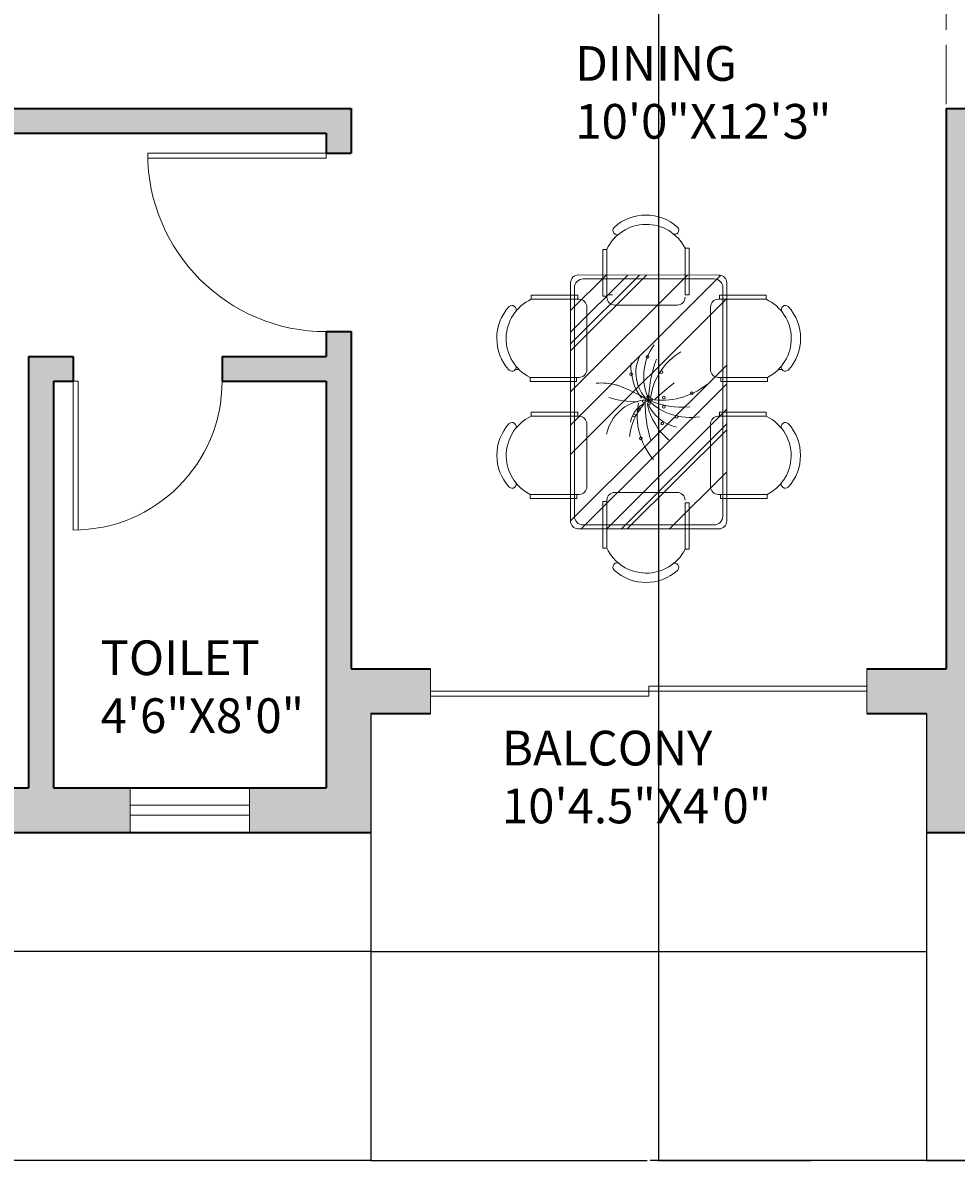
# Model space of a CAD drawing. Units: inches. Extents: x 2540 to 3167, y 3083 to 4007.
# Tile 2 of 15: x 2740 to 2929, y 3083 to 3313. Entities that reach past the tile are written whole.
import ezdxf

# ---------------------------------------------------------------- set-up
doc = ezdxf.new("R2010")
doc.units = ezdxf.units.IN
doc.linetypes.add('ACAD_ISO02W100', pattern=[15, 12, -3])
for name, color, linetype, lineweight in [('A-ANNO-DIMS', 2, 'Continuous', 18), ('A-AREA-IDEN', 7, 'Continuous', 18), ('A-DOOR', 4, 'Continuous', 18), ('A-FLOR-EDGE', 7, 'Continuous', 25), ('A-FURN', 8, 'Continuous', 13), ('A-GLAZ', 4, 'Continuous', 18)]:
    doc.layers.add(name, color=color, linetype=linetype, lineweight=lineweight)
for name, color, linetype, lineweight, true_color in [('A-WALL', 143, 'Continuous', 35, 0x7aafdf), ('A-WALL-OVHD', 143, 'ACAD_ISO02W100', 18, 0x7aafdf), ('A-WALL-PATT', 143, 'Continuous', 13, 0x7aafdf)]:
    doc.layers.add(name, color=color, linetype=linetype, lineweight=lineweight, true_color=true_color)
doc.styles.get("Standard").update_dxf_attribs({"font": 'arial.ttf'})
doc.dimstyles.get("Standard").update_dxf_attribs({"dimtxt": 0.18, "dimasz": 0.18, "dimexe": 0.18, "dimexo": 0.0625, "dimgap": 0.09, "dimtad": 0, "dimtih": 1, "dimtoh": 1, "dimdec": 4, "dimzin": 0, "dimdsep": 46, "dimtxsty": 'Standard', "dimcen": 0.09, "dimadec": 0, "dimazin": 0, "dimtfac": 1, "dimtdec": 4, "dimtofl": 0, "dimtmove": 0, "dimatfit": 3, "dimfxl": 1, "dimtolj": 1, "dimtzin": 0, "dimarcsym": 0})

# ---------------------------------------------------------------- blocks, each defined once
blk = doc.blocks.new('A$C6327331B')
for p, q in [((790.8, 678.3), (790.8, 696.4)), ((790.8, 678.3), (790.8, 696.4)), ((1381.3, 692.8), (1381.3, 686.2)), ((1381.3, 692.8), (1381.3, 686.2)), ((410.1, 615.8), (410, 377)), ((410.1, 615.8), (410, 377)), ((431.6, 615.8), (410.1, 615.8)), ((431.6, 615.8), (410.1, 615.8)), ((431.4, 376.9), (431.6, 615.8)), ((431.4, 376.9), (431.6, 615.8)), ((831.4, 382.9), (831.6, 621.7)), ((831.4, 382.9), (831.6, 621.7)), ((831.6, 621.7), (853, 621.7)), ((831.6, 621.7), (853, 621.7)), ((853, 621.7), (852.9, 382.9)), ((853, 621.7), (852.9, 382.9)), ((1009.3, 615.5), (1009.2, 376.7)), ((1009.3, 615.5), (1009.2, 376.7)), ((1030.7, 615.5), (1009.3, 615.5)), ((1030.7, 615.5), (1009.3, 615.5)), ((1030.6, 376.6), (1030.7, 615.5)), ((1030.6, 376.6), (1030.7, 615.5)), ((1430.6, 382.6), (1430.7, 621.4)), ((1430.6, 382.6), (1430.7, 621.4)), ((1430.7, 621.4), (1452.2, 621.4)), ((1430.7, 621.4), (1452.2, 621.4)), ((1452.2, 621.4), (1452, 382.6)), ((1452.2, 621.4), (1452, 382.6)), ((431.5, 571.8), (431.4, 370.8)), ((431.5, 571.8), (431.4, 370.8)), ((831.4, 370.6), (831.5, 571.6)), ((831.4, 370.6), (831.5, 571.6)), ((1030.7, 571.5), (1030.6, 370.5)), ((1030.7, 571.5), (1030.6, 370.5)), ((1430.6, 370.3), (1430.7, 571.3)), ((1430.6, 370.3), (1430.7, 571.3)), ((347.5, 414), (831.5, 413.8)), ((347.5, 414), (831.5, 413.8)), ((1226.3, -386.4), (428, 414)), ((1226.3, -386.4), (428, 414)), ((1567.1, -386.6), (768.8, 413.8)), ((1567.1, -386.6), (768.8, 413.8)), ((831.5, 413.8), (1567.5, 413.4)), ((1607.1, -331.3), (864.1, 413.8)), ((1607.1, -331.3), (864.1, 413.8)), ((1607.2, -200.8), (994.4, 413.7)), ((1607.2, -200.8), (994.4, 413.7)), ((1009.2, 413.7), (1567.5, 413.4)), ((1607.2, -125.5), (1069.5, 413.7)), ((1607.2, -125.5), (1069.5, 413.7)), ((1607.2, -95.4), (1099.6, 413.6)), ((1607.2, -95.4), (1099.6, 413.6)), ((1607.3, 120.5), (1315.1, 413.5)), ((1607.3, 120.5), (1315.1, 413.5)), ((1415.7, 413.4), (1415.7, 413.5)), ((1415.7, 413.4), (1415.7, 413.5)), ((307.1, -346), (307.5, 374)), ((307.1, -346), (307.5, 374)), ((1075.9, -386.3), (308.5, 383.1)), ((1075.9, -386.3), (308.5, 383.1)), ((372.5, 394), (831.4, 393.8)), ((372.5, 394), (1009.2, 393.7)), ((410, 377), (431.4, 376.9)), ((410, 377), (431.4, 376.9)), ((852.9, 382.9), (831.4, 382.9)), ((852.9, 382.9), (831.4, 382.9)), ((1009.2, 393.7), (1542.5, 393.4)), ((1009.2, 376.7), (1030.6, 376.6)), ((1009.2, 376.7), (1030.6, 376.6)), ((1452, 382.6), (1430.6, 382.6)), ((1452, 382.6), (1430.6, 382.6)), ((1607.5, 373.4), (1607.1, -346.6)), ((1607.5, 373.4), (1607.1, -346.6)), ((327.1, -321), (327.5, 349)), ((471.4, 330.8), (791.4, 330.6)), ((471.4, 330.8), (791.4, 330.6)), ((1070.6, 330.5), (1390.6, 330.3)), ((1070.6, 330.5), (1390.6, 330.3)), ((1587.5, 348.4), (1587.1, -321.6)), ((169.9, 221.5), (408.7, 221.6)), ((169.9, 221.5), (408.7, 221.6)), ((169.9, 200.1), (169.9, 221.5)), ((169.9, 200.1), (169.9, 221.5)), ((408.7, 200.2), (169.9, 200.1)), ((408.7, 200.2), (169.9, 200.1)), ((905.5, -386.3), (307.4, 213.5)), ((905.5, -386.3), (307.4, 213.5)), ((408.7, 221.6), (408.7, 200.2)), ((408.7, 221.6), (408.7, 200.2)), ((1473.3, 221.6), (1473.3, 200.2)), ((1473.3, 221.6), (1473.3, 200.2)), ((1712.1, 221.5), (1473.3, 221.6)), ((1712.1, 221.5), (1473.3, 221.6)), ((1473.3, 200.2), (1712.1, 200.1)), ((1473.3, 200.2), (1712.1, 200.1)), ((1712.1, 200.1), (1712.1, 221.5)), ((1712.1, 200.1), (1712.1, 221.5)), ((461.2, -159.8), (461, 160.2)), ((461.2, -159.8), (461, 160.2)), ((1420.8, -159.8), (1420.9, 160.2)), ((1420.8, -159.8), (1420.9, 160.2)), ((695.1, -386.2), (307.3, 2.7)), ((695.1, -386.2), (307.3, 2.7)), ((44.6, -20.2), (44.5, -20.1)), ((44.6, -20.2), (44.5, -20.1)), ((660, -386.1), (307.3, -32.5)), ((660, -386.1), (307.3, -32.5)), ((1837.4, -20.2), (1837.5, -20.1)), ((1837.4, -20.2), (1837.5, -20.1)), ((599.8, -386.1), (307.2, -92.7)), ((599.8, -386.1), (307.2, -92.7)), ((408.7, -193.6), (408.7, -172.1)), ((408.7, -193.6), (408.7, -172.1)), ((415.1, -199.8), (176.2, -199.9)), ((415.1, -199.8), (176.2, -199.9)), ((176.2, -199.9), (176.2, -221.3)), ((176.2, -199.9), (176.2, -221.3)), ((176.2, -221.3), (415.1, -221.2)), ((176.2, -221.3), (415.1, -221.2)), ((220.2, -199.9), (421.2, -199.8)), ((220.2, -199.9), (421.2, -199.8)), ((489.6, -386), (307.2, -203.2)), ((489.6, -386), (307.2, -203.2)), ((415.1, -221.2), (415.1, -199.8)), ((415.1, -221.2), (415.1, -199.8)), ((1661.8, -199.9), (1460.8, -199.8)), ((1661.8, -199.9), (1460.8, -199.8)), ((1466.9, -221.2), (1466.9, -199.8)), ((1466.9, -221.2), (1466.9, -199.8)), ((1466.9, -199.8), (1705.7, -199.9)), ((1466.9, -199.8), (1705.7, -199.9)), ((1705.7, -221.3), (1466.9, -221.2)), ((1705.7, -221.3), (1466.9, -221.2)), ((1705.7, -199.9), (1705.7, -221.3)), ((1705.7, -199.9), (1705.7, -221.3)), ((410.1, -587.7), (410, -348.9)), ((410.1, -587.7), (410, -348.9)), ((410, -348.9), (431.4, -348.9)), ((410, -348.9), (431.4, -348.9)), ((431.5, -543.7), (431.4, -342.7)), ((431.5, -543.7), (431.4, -342.7)), ((431.4, -348.9), (431.6, -587.7)), ((431.4, -348.9), (431.6, -587.7)), ((471.4, -302.7), (791.4, -302.5)), ((471.4, -302.7), (791.4, -302.5)), ((831.4, -342.5), (831.5, -543.5)), ((831.4, -342.5), (831.5, -543.5)), ((1009.2, -348.6), (1030.6, -348.5)), ((1009.2, -348.6), (1030.6, -348.5)), ((1009.3, -587.4), (1009.2, -348.6)), ((1009.3, -587.4), (1009.2, -348.6)), ((1030.7, -543.4), (1030.6, -342.4)), ((1030.7, -543.4), (1030.6, -342.4)), ((1030.6, -348.5), (1030.7, -587.4)), ((1030.6, -348.5), (1030.7, -587.4)), ((1070.6, -302.4), (1390.6, -302.2)), ((1070.6, -302.4), (1390.6, -302.2)), ((1430.6, -342.2), (1430.7, -543.2)), ((1430.6, -342.2), (1430.7, -543.2)), ((1567.1, -386.6), (347.1, -386)), ((1567.1, -386.6), (347.1, -386)), ((1542.1, -366.6), (372.1, -366)), ((831.4, -354.8), (831.6, -593.6)), ((831.4, -354.8), (831.6, -593.6)), ((852.9, -354.8), (831.4, -354.8)), ((852.9, -354.8), (831.4, -354.8)), ((831.5, -385.7), (864.1, -385.7)), ((831.5, -385.7), (864.1, -385.7)), ((853, -593.6), (852.9, -354.8)), ((853, -593.6), (852.9, -354.8)), ((1415.7, -385.3), (1415.7, -385.4)), ((1415.7, -385.3), (1415.7, -385.4)), ((1430.6, -354.5), (1430.7, -593.3)), ((1430.6, -354.5), (1430.7, -593.3)), ((1452, -354.5), (1430.6, -354.5)), ((1452, -354.5), (1430.6, -354.5)), ((1452.2, -593.3), (1452, -354.5)), ((1452.2, -593.3), (1452, -354.5)), ((431.6, -587.7), (410.1, -587.7)), ((431.6, -587.7), (410.1, -587.7)), ((831.6, -593.6), (853, -593.6)), ((831.6, -593.6), (853, -593.6)), ((1030.7, -587.4), (1009.3, -587.4)), ((1030.7, -587.4), (1009.3, -587.4)), ((1430.7, -593.3), (1452.2, -593.3)), ((1430.7, -593.3), (1452.2, -593.3)), ((790.8, -650.2), (790.8, -668.4)), ((790.8, -650.2), (790.8, -668.4)), ((1381.3, -664.7), (1381.3, -658.1)), ((1381.3, -664.7), (1381.3, -658.1))]:
    blk.add_line(p, q)
for centre, radius, start, end in [((631.5, 550.5), 241.3, 47.46915, 132.47205), ((631.5, 550.5), 241.3, 47.46915, 132.47205), ((1230.7, 550.2), 241.3, 47.46915, 132.47205), ((1230.7, 550.2), 241.3, 47.46915, 132.47205), ((633, 521.6), 222.4, 26.76564, 154.93691), ((633, 521.6), 222.4, 26.76564, 154.93691), ((484.3, 714.2), 21.2, 137.64965, 300.34124), ((484.3, 714.2), 21.2, 137.64965, 300.34124), ((779, 714), 21.2, 239.59996, 42.29154), ((779, 714), 21.2, 239.59996, 42.29154), ((1232.2, 521.3), 222.4, 84.42654, 154.93691), ((1232.2, 521.3), 222.4, 84.42654, 154.93691), ((1083.4, 713.9), 21.2, 137.64965, 300.34124), ((1083.4, 713.9), 21.2, 137.64965, 300.34124), ((1232.2, 521.3), 222.4, 26.76564, 84.42654), ((1232.2, 521.3), 222.4, 26.76564, 84.42654), ((1378.1, 713.7), 21.2, 239.59996, 42.29154), ((1378.1, 713.7), 21.2, 239.59996, 42.29154), ((347.5, 374), 40, 89.9706, 179.9706), ((347.5, 374), 40, 89.9706, 179.9706), ((1567.5, 373.4), 40, 359.9706, 89.9706), ((1567.5, 373.4), 40, 359.9706, 89.9706), ((372.5, 349), 45, 89.9706, 179.9706), ((471.4, 370.8), 40, 179.9706, 269.9706), ((471.4, 370.8), 40, 179.9706, 269.9706), ((791.4, 370.6), 40, 269.9706, 359.9706), ((791.4, 370.6), 40, 269.9706, 359.9706), ((1070.6, 370.5), 40, 179.9706, 269.9706), ((1070.6, 370.5), 40, 179.9706, 269.9706), ((1390.6, 370.3), 40, 269.9706, 359.9706), ((1390.6, 370.3), 40, 269.9706, 359.9706), ((1542.5, 348.4), 45, 359.9706, 89.9706), ((574.1, 79.9), 374.6, 351.24958, 38.23328), ((912.6, 235.7), 6.91, 0, 180), ((912.6, 235.7), 6.91, 180, 0), ((737.8, 225), 299.2, 314.48606, 9.37622), ((270.2, 1.6), 222.4, 116.82445, 244.99571), ((270.2, 1.6), 222.4, 116.82445, 244.99571), ((421, 160.2), 40, 0.0294, 90.0294), ((421, 160.2), 40, 0.0294, 90.0294), ((983.2, 350.8), 331, 211.31505, 262.13779), ((586.4, 182.9), 398.1, 335.08876, 5.96372), ((1460.9, 160.2), 40, 89.9706, 179.9706), ((1460.9, 160.2), 40, 89.9706, 179.9706), ((1611.7, 1.6), 222.4, 295.00429, 63.17555), ((1611.7, 1.6), 222.4, 295.00429, 63.17555), ((241.3, 0.1), 241.3, 137.52795, 222.53085), ((77.6, 147.4), 21.2, 329.65876, 132.35035), ((77.6, 147.4), 21.2, 329.65876, 132.35035), ((2460.3, 1443.6), 2062.1, 219.04877, 222.6799), ((873.8, 207.8), 219.3, 294.09558, 346.29534), ((897.1, 334.6), 335.6, 283.04524, 319.77663), ((1033, 155.9), 6.91, 0, 180), ((1033, 155.9), 6.91, 180, 0), ((1804.4, 147.4), 21.2, 47.64965, 210.34124), ((1804.4, 147.4), 21.2, 47.64965, 210.34124), ((1640.7, 0.1), 241.3, 317.46915, 42.47205), ((1640.7, 0.1), 241.3, 317.46915, 42.47205), ((805, 79.9), 6.91, 0, 180), ((805, 79.9), 6.91, 180, 0), ((934.8, 91.3), 6.91, 0, 180), ((934.8, 91.3), 6.91, 180, 0), ((982.3, 91.3), 6.91, 0, 180), ((982.3, 91.3), 6.91, 180, 0), ((1067.8, 83.7), 6.91, 0, 180), ((1067.8, 83.7), 6.91, 180, 0), ((826.9, 258.5), 270.1, 233.32313, 295.76326), ((725.8, 7.7), 6.91, 0, 180), ((725.8, 7.7), 6.91, 180, 0), ((807.8, 143), 194.5, 242.99086, 315.91017), ((985.1, 750.7), 739.8, 250.5249, 267.82437), ((1747.6, -469.5), 933.6, 148.98728, 160.36101), ((931.7, 11.5), 6.91, 0, 180), ((931.7, 11.5), 6.91, 180, 0), ((944.3, 26.7), 6.91, 0, 180), ((944.3, 26.7), 6.91, 180, 0), ((947.5, 3.9), 6.91, 0, 180), ((947.5, 3.9), 6.91, 180, 0), ((970.7, 574.8), 578.8, 268.32856, 288.729), ((966.5, 15.3), 6.91, 0, 180), ((966.5, 15.3), 6.91, 180, 0), ((1030.3, 292.7), 337.4, 258.55155, 310.98153), ((776.7, 191.6), 268.2, 265.87406, 306.95584), ((392.7, -33), 564.4, 343.85612, 359.11051), ((953.8, -11.3), 6.91, 0, 180), ((953.8, -11.3), 6.91, 180, 0), ((1167.7, 15.7), 221.9, 186.99045, 258.02836), ((1090.6, 62.7), 145.4, 208.89012, 258.45792), ((1166.2, 212.9), 298.2, 228.7581, 263.8624), ((995, -34.1), 6.91, 0, 180), ((995, -34.1), 6.91, 180, 0), ((1026.7, -60.7), 6.91, 0, 180), ((1143.8, -26.5), 6.91, 0, 180), ((1143.8, -26.5), 6.91, 180, 0), ((814.5, -75.9), 6.91, 0, 180), ((814.5, -75.9), 6.91, 180, 0), ((1026.7, -60.7), 6.91, 180, 0), ((79, -146.7), 22.5, 226.37763, 29.88821), ((79, -146.7), 22.5, 226.37763, 29.88821), ((421.2, -159.8), 40, 270.0294, 0.0294), ((421.2, -159.8), 40, 270.0294, 0.0294), ((1112.9, -226), 252.6, 162.94564, 186.48138), ((1460.8, -159.8), 40, 179.9706, 269.9706), ((1460.8, -159.8), 40, 179.9706, 269.9706), ((1803, -146.7), 22.5, 150.11179, 313.62237), ((1803, -146.7), 22.5, 150.11179, 313.62237), ((347.1, -346), 40, 179.9706, 269.9706), ((347.1, -346), 40, 179.9706, 269.9706), ((372.1, -321), 45, 179.9706, 269.9706), ((471.4, -342.7), 40, 90.0294, 180.0294), ((471.4, -342.7), 40, 90.0294, 180.0294), ((791.4, -342.5), 40, 0.0294, 90.0294), ((791.4, -342.5), 40, 0.0294, 90.0294), ((1070.6, -342.4), 40, 90.0294, 180.0294), ((1070.6, -342.4), 40, 90.0294, 180.0294), ((1390.6, -342.2), 40, 0.0294, 90.0294), ((1390.6, -342.2), 40, 0.0294, 90.0294), ((1542.1, -321.6), 45, 269.9706, 359.9706), ((1567.1, -346.6), 40, 269.9706, 359.9706), ((1567.1, -346.6), 40, 269.9706, 359.9706), ((633, -493.5), 222.4, 205.06309, 333.23436), ((633, -493.5), 222.4, 205.06309, 333.23436), ((1232.2, -493.2), 222.4, 205.06309, 275.57346), ((1232.2, -493.2), 222.4, 205.06309, 275.57346), ((1232.2, -493.2), 222.4, 275.57346, 333.23436), ((1232.2, -493.2), 222.4, 275.57346, 333.23436), ((484.3, -686.1), 21.2, 59.65876, 222.35035), ((484.3, -686.1), 21.2, 59.65876, 222.35035), ((779, -686), 21.2, 317.70846, 120.40004), ((779, -686), 21.2, 317.70846, 120.40004), ((1083.4, -685.8), 21.2, 59.65876, 222.35035), ((1083.4, -685.8), 21.2, 59.65876, 222.35035), ((1378.1, -685.6), 21.2, 317.70846, 120.40004), ((1378.1, -685.6), 21.2, 317.70846, 120.40004), ((631.5, -522.4), 241.3, 227.52795, 312.53085), ((631.5, -522.4), 241.3, 227.52795, 312.53085), ((1230.7, -522.1), 241.3, 227.52795, 312.53085), ((1230.7, -522.1), 241.3, 227.52795, 312.53085)]:
    blk.add_arc(centre, radius, start, end)
at = {"width": 0.8, "flags": 9}
for tag in ['XSIZE', 'YSIZE']:
    blk.add_attdef(tag, (945.2, 11.4), '', height=0.23, rotation=180, dxfattribs=at)
blk = doc.blocks.new('DOOR-SWING-36IN')
for p, q in [((36, 0), (0, 0)), ((36, 1), (0.01, 1)), ((36, 1), (36, 0))]:
    blk.add_line(p, q)
blk.add_arc((36, 0), 36, 90, 180)
blk = doc.blocks.new('DOOR-SWING-30IN')
for p, q in [((0, 0), (0, 30)), ((1, 0), (1, 29.98)), ((0, 0), (1, 0))]:
    blk.add_line(p, q)
blk.add_arc((0, 0), 30, 0, 90)
blk = doc.blocks.new('WIN-24IN')
for p, q in [((0, 24), (9, 24)), ((3.5, 0), (3.5, 24)), ((5.5, 0), (5.5, 24)), ((0, 0), (9, 0))]:
    blk.add_line(p, q)
blk = doc.blocks.new('*D44')
at = {"layer": 'A-ANNO-DIMS', "color": 0, "lineweight": -2, "transparency": 16777216}
for p, q in [((2771.45, 3964.71), (2540.23, 3964.71)), ((2540.41, 3964.53), (2540.41, 3545.4)), ((2540.41, 3125.89), (2540.41, 3545.03)), ((2810.45, 3125.71), (2540.23, 3125.71))]:
    blk.add_line(p, q, dxfattribs=at)
at = {"layer": 'A-ANNO-DIMS', "color": 0, "transparency": 16777216}
for points in [[(2540.38, 3964.53), (2540.44, 3964.53), (2540.41, 3964.71)], [(2540.38, 3125.89), (2540.44, 3125.89), (2540.41, 3125.71)]]:
    blk.add_solid(points, dxfattribs=at)
at = {"layer": 'Defpoints', "color": 0, "transparency": 16777216}
for p in [(2540.41, 3964.71), (2771.51, 3964.71), (2810.51, 3125.71)]:
    blk.add_point(p, dxfattribs=at)
at = {"layer": 'A-ANNO-DIMS', "color": 0, "transparency": 16777216, "insert": (2540.41, 3545.21), "char_height": 0.18, "attachment_point": 5}
blk.add_mtext('\\A1;839', dxfattribs=at)
blk = doc.blocks.new('*D45')
at = {"layer": 'A-ANNO-DIMS', "color": 0, "lineweight": -2, "transparency": 16777216}
for p, q in [((2612.51, 3149.65), (2612.51, 3083.43)), ((2810.51, 3125.65), (2810.51, 3083.43)), ((2612.69, 3083.61), (2711.23, 3083.61)), ((2810.33, 3083.61), (2711.79, 3083.61))]:
    blk.add_line(p, q, dxfattribs=at)
at = {"layer": 'A-ANNO-DIMS', "color": 0, "transparency": 16777216}
for points in [[(2612.69, 3083.64), (2612.69, 3083.58), (2612.51, 3083.61)], [(2810.33, 3083.64), (2810.33, 3083.58), (2810.51, 3083.61)]]:
    blk.add_solid(points, dxfattribs=at)
at = {"layer": 'Defpoints', "color": 0, "transparency": 16777216}
for p in [(2612.51, 3149.71), (2810.51, 3125.71), (2810.51, 3083.61)]:
    blk.add_point(p, dxfattribs=at)
at = {"layer": 'A-ANNO-DIMS', "color": 0, "transparency": 16777216, "insert": (2711.51, 3083.61), "char_height": 0.18, "attachment_point": 5}
blk.add_mtext('\\A1;198', dxfattribs=at)
blk = doc.blocks.new('*D46')
at = {"layer": 'A-ANNO-DIMS', "color": 0, "lineweight": -2, "transparency": 16777216}
for p, q in [((2810.51, 3125.65), (2810.51, 3083.43)), ((2922.51, 3125.65), (2922.51, 3083.43)), ((2810.69, 3083.61), (2866.23, 3083.61)), ((2922.33, 3083.61), (2866.79, 3083.61))]:
    blk.add_line(p, q, dxfattribs=at)
at = {"layer": 'A-ANNO-DIMS', "color": 0, "transparency": 16777216}
for points in [[(2810.69, 3083.64), (2810.69, 3083.58), (2810.51, 3083.61)], [(2922.33, 3083.64), (2922.33, 3083.58), (2922.51, 3083.61)]]:
    blk.add_solid(points, dxfattribs=at)
at = {"layer": 'Defpoints', "color": 0, "transparency": 16777216}
for p in [(2810.51, 3125.71), (2922.51, 3125.71), (2922.51, 3083.61)]:
    blk.add_point(p, dxfattribs=at)
at = {"layer": 'A-ANNO-DIMS', "color": 0, "transparency": 16777216, "insert": (2866.51, 3083.61), "char_height": 0.18, "attachment_point": 5}
blk.add_mtext('\\A1;112', dxfattribs=at)
blk = doc.blocks.new('*D47')
at = {"layer": 'A-ANNO-DIMS', "color": 0, "lineweight": -2, "transparency": 16777216}
for p, q in [((3124.51, 3149.65), (3124.51, 3083.43)), ((2922.51, 3125.65), (2922.51, 3083.43)), ((2922.69, 3083.61), (3023.22, 3083.61)), ((3124.33, 3083.61), (3023.8, 3083.61))]:
    blk.add_line(p, q, dxfattribs=at)
at = {"layer": 'A-ANNO-DIMS', "color": 0, "transparency": 16777216}
for points in [[(2922.69, 3083.64), (2922.69, 3083.58), (2922.51, 3083.61)], [(3124.33, 3083.64), (3124.33, 3083.58), (3124.51, 3083.61)]]:
    blk.add_solid(points, dxfattribs=at)
at = {"layer": 'Defpoints', "color": 0, "transparency": 16777216}
for p in [(3124.51, 3149.71), (2922.51, 3125.71), (3124.51, 3083.61)]:
    blk.add_point(p, dxfattribs=at)
at = {"layer": 'A-ANNO-DIMS', "color": 0, "transparency": 16777216, "insert": (3023.51, 3083.61), "char_height": 0.18, "attachment_point": 5}
blk.add_mtext('\\A1;202', dxfattribs=at)
blk = doc.blocks.new('*D55')
at = {"layer": 'A-ANNO-DIMS', "color": 0, "lineweight": -2, "transparency": 16777216}
for p, q in [((2868.51, 3564.65), (2868.51, 3083.43)), ((2930.51, 3543.65), (2930.51, 3083.43)), ((2868.69, 3083.61), (2899.29, 3083.61)), ((2930.33, 3083.61), (2899.73, 3083.61))]:
    blk.add_line(p, q, dxfattribs=at)
at = {"layer": 'A-ANNO-DIMS', "color": 0, "transparency": 16777216}
for points in [[(2868.69, 3083.64), (2868.69, 3083.58), (2868.51, 3083.61)], [(2930.33, 3083.64), (2930.33, 3083.58), (2930.51, 3083.61)]]:
    blk.add_solid(points, dxfattribs=at)
at = {"layer": 'Defpoints', "color": 0, "transparency": 16777216}
for p in [(2868.51, 3564.71), (2930.51, 3543.71), (2930.51, 3083.61)]:
    blk.add_point(p, dxfattribs=at)
at = {"layer": 'A-ANNO-DIMS', "color": 0, "transparency": 16777216, "insert": (2899.51, 3083.61), "char_height": 0.18, "attachment_point": 5}
blk.add_mtext('\\A1;62', dxfattribs=at)

msp = doc.modelspace()

# ---------------------------------------------------------------- hatches: boundary and pattern name
at = {"layer": 'A-WALL-PATT'}
h = msp.add_hatch(color=256, dxfattribs=at)
h.dxf.hatch_style = 1
h.paths.add_polyline_path([(2805.51, 3803.71), (2800.51, 3803.71), (2800.51, 3799.71), (2621.51, 3799.71), (2621.51, 3823.71), (2612.51, 3823.71), (2612.51, 3794.71), (2636.51, 3794.71), (2636.51, 3782.71), (2645.51, 3782.71), (2645.51, 3794.71), (2805.51, 3794.71)])
h.paths.add_polyline_path([(2810.51, 3564.71), (2868.51, 3564.71), (2868.51, 3627.71), (2872.51, 3627.71), (2872.51, 3636.71), (2864.51, 3636.71), (2864.51, 3674.71), (2797.51, 3674.71), (2797.51, 3669.71), (2801.51, 3669.71), (2801.51, 3628.63), (2806.51, 3628.63), (2806.51, 3669.71), (2859.51, 3669.71), (2859.51, 3573.71), (2806.51, 3573.71), (2806.51, 3598.63), (2801.51, 3598.63), (2801.51, 3549.71), (2645.51, 3549.71), (2645.51, 3573.71), (2636.51, 3573.71), (2636.51, 3516.71), (2645.51, 3516.71), (2645.51, 3540.71), (2801.51, 3540.71), (2801.51, 3504.71), (2801.51, 3500.71), (2806.51, 3500.71), (2806.51, 3504.71), (2859.51, 3504.71), (2859.51, 3420.71), (2806.51, 3420.71), (2806.51, 3470.71), (2801.51, 3470.71), (2801.51, 3420.71), (2797.51, 3420.71), (2797.51, 3415.71), (2864.51, 3415.71), (2864.51, 3453.71), (2868.51, 3453.71), (2868.51, 3513.71), (2810.51, 3513.71)])
h.paths.add_polyline_path([(2645.51, 3415.71), (2761.51, 3415.71), (2761.51, 3420.71), (2645.51, 3420.71), (2645.51, 3444.71), (2636.51, 3444.71), (2636.51, 3403.71), (2645.51, 3403.71)])
h.paths.add_polyline_path([(2645.51, 3307.71), (2636.51, 3307.71), (2636.51, 3295.71), (2612.51, 3295.71), (2612.51, 3149.71), (2645.51, 3149.71), (2645.51, 3158.71), (2621.51, 3158.71), (2621.51, 3290.71), (2801.51, 3290.71), (2801.51, 3286.71), (2806.51, 3286.71), (2806.51, 3295.71), (2645.51, 3295.71)])
h.paths.add_polyline_path([(2762.01, 3158.71), (2746.51, 3158.71), (2746.51, 3240.71), (2750.51, 3240.71), (2750.51, 3245.71), (2741.51, 3245.71), (2741.51, 3158.71), (2717.51, 3158.71), (2717.51, 3149.71), (2762.01, 3149.71)], flags=17)
h.paths.add_polyline_path([(2810.51, 3173.71), (2822.51, 3173.71), (2822.51, 3182.71), (2806.51, 3182.71), (2806.51, 3250.71), (2801.51, 3250.71), (2801.51, 3245.71), (2780.51, 3245.71), (2780.51, 3240.71), (2801.51, 3240.71), (2801.51, 3158.71), (2786.01, 3158.71), (2786.01, 3149.71), (2810.51, 3149.71)])
h.paths.add_polyline_path([(2931.51, 3290.71), (2935.51, 3290.71), (2935.51, 3295.71), (2926.51, 3295.71), (2926.51, 3182.71), (2910.51, 3182.71), (2910.51, 3173.71), (2922.51, 3173.71), (2922.51, 3149.71), (2987.51, 3149.71), (2987.51, 3158.71), (2931.51, 3158.71)])
h.paths.add_polyline_path([(3124.51, 3295.71), (3086.51, 3295.71), (3018.51, 3295.71), (3018.51, 3290.71), (3115.51, 3290.71), (3115.51, 3158.71), (3059.51, 3158.71), (3059.51, 3149.71), (3124.51, 3149.71)])
h.paths.add_polyline_path([(2988.51, 3295.71), (2984.51, 3295.71), (2984.51, 3349.71), (3086.51, 3349.71), (3086.51, 3320.71), (3124.51, 3320.71), (3124.51, 3354.71), (3071.51, 3354.71), (3071.51, 3358.71), (3062.51, 3358.71), (3062.51, 3354.71), (2979.51, 3354.71), (2979.51, 3295.71), (2971.51, 3295.71), (2971.51, 3290.71), (2988.51, 3290.71)])
h.paths.add_polyline_path([(3095.51, 3325.71), (3095.51, 3349.71), (3119.51, 3349.71), (3119.51, 3325.71)], flags=16)
h.paths.add_polyline_path([(3124.51, 3462.71), (3071.51, 3462.71), (3071.51, 3627.71), (3124.51, 3627.71), (3124.51, 3693.71), (3095.51, 3693.71), (3095.51, 3702.71), (3086.51, 3702.71), (3086.51, 3684.71), (3086.51, 3636.71), (2930.51, 3636.71), (2930.51, 3768.71), (2934.51, 3768.71), (2934.51, 3773.71), (2930.51, 3773.71), (2925.51, 3773.71), (2925.51, 3730.71), (2864.51, 3730.71), (2864.51, 3760.71), (2859.51, 3760.71), (2859.51, 3725.71), (2925.51, 3725.71), (2925.51, 3636.71), (2908.51, 3636.71), (2908.51, 3627.71), (3062.51, 3627.71), (3062.51, 3543.71), (2930.51, 3543.71), (2930.51, 3534.71), (2993.51, 3534.71), (2993.51, 3516.71), (3002.51, 3516.71), (3002.51, 3534.71), (3062.51, 3534.71), (3062.51, 3462.71), (3002.51, 3462.71), (3002.51, 3480.71), (2993.51, 3480.71), (2993.51, 3462.71), (2916.51, 3462.71), (2916.51, 3453.71), (2926.51, 3453.71), (2926.51, 3361.71), (2859.51, 3361.71), (2859.51, 3338.71), (2864.51, 3338.71), (2864.51, 3356.71), (2926.51, 3356.71), (2926.51, 3338.71), (2931.51, 3338.71), (2931.51, 3453.71), (3062.51, 3453.71), (3062.51, 3448.21), (3071.51, 3448.21), (3071.51, 3453.71), (3124.51, 3453.71)])

# ---------------------------------------------------------------- linework, layer by layer
at = {"layer": 'A-DOOR'}
for p, q in [((2822.51, 3173.71), (2822.51, 3182.71)), ((2910.51, 3173.71), (2910.51, 3182.71)), ((2910.51, 3178.21), (2822.51, 3178.21)), ((2866.51, 3177.21), (2822.51, 3177.21)), ((2910.51, 3179.21), (2866.51, 3179.21)), ((2866.51, 3179.21), (2866.51, 3177.21))]:
    msp.add_line(p, q, dxfattribs=at)
at = {"layer": 'A-FLOR-EDGE'}
for p, q in [((2810.51, 3173.71), (2810.51, 3125.71)), ((2922.51, 3173.71), (2922.51, 3125.71)), ((2810.51, 3125.71), (2922.51, 3125.71))]:
    msp.add_line(p, q, dxfattribs=at)
at = {"layer": 'A-WALL'}
for p, q in [((2645.51, 3295.71), (2806.51, 3295.71)), ((2806.51, 3295.71), (2806.51, 3286.71)), ((2926.51, 3295.71), (2935.51, 3295.71)), ((2926.51, 3295.71), (2926.51, 3182.71)), ((2621.51, 3290.71), (2801.51, 3290.71)), ((2801.51, 3290.71), (2801.51, 3286.71)), ((2801.51, 3286.71), (2806.51, 3286.71)), ((2801.51, 3250.71), (2806.51, 3250.71)), ((2801.51, 3250.71), (2801.51, 3245.71)), ((2806.51, 3250.71), (2806.51, 3182.71)), ((2741.51, 3245.71), (2741.51, 3158.71)), ((2741.51, 3245.71), (2750.51, 3245.71)), ((2750.51, 3245.71), (2750.51, 3240.71)), ((2780.51, 3245.71), (2780.51, 3240.71)), ((2780.51, 3245.71), (2801.51, 3245.71)), ((2746.51, 3240.71), (2746.51, 3158.71)), ((2746.51, 3240.71), (2750.51, 3240.71)), ((2780.51, 3240.71), (2801.51, 3240.71)), ((2801.51, 3240.71), (2801.51, 3158.71)), ((2806.51, 3182.71), (2822.51, 3182.71)), ((2910.51, 3182.71), (2926.51, 3182.71)), ((2810.51, 3173.71), (2822.51, 3173.71)), ((2910.51, 3173.71), (2922.51, 3173.71)), ((2621.51, 3158.71), (2741.51, 3158.71)), ((2746.51, 3158.71), (2801.51, 3158.71)), ((2612.51, 3149.71), (2810.51, 3149.71)), ((2922.51, 3149.71), (3124.51, 3149.71))]:
    msp.add_line(p, q, dxfattribs=at)
at = {"layer": 'A-WALL-OVHD'}
msp.add_line((2926.51, 3338.56), (2926.51, 3295.71), dxfattribs=at)

# ---------------------------------------------------------------- block references
at = {"layer": 'A-DOOR', "extrusion": (0, 0, -1), "zscale": -1, "rotation": 180}
for name, p in [('DOOR-SWING-36IN', (-2765.51, 3286.71)), ('DOOR-SWING-30IN', (-2750.51, 3240.71))]:
    msp.add_blockref(name, p, dxfattribs=at)
at = {"layer": 'A-FURN', "xscale": 0.0393700787401575, "yscale": 0.0393700787401575, "zscale": 0.0393700787401575, "rotation": 270}
msp.add_blockref('A$C6327331B', (2865.96, 3274.23), dxfattribs=at)
at = {"layer": 'A-GLAZ', "rotation": 270.0000000000064}
msp.add_blockref('WIN-24IN', (2762.01, 3158.71), dxfattribs=at)

# ---------------------------------------------------------------- texts
at = {"layer": 'A-AREA-IDEN', "char_height": 7, "attachment_point": 1}
for s, width, insert in [('DINING\\P10\'0"X12\'3"', 74.1323, (2851.72, 3308.29)), ('TOILET\\P4\'6"X8\'0"', 75.6369, (2756.01, 3188.45)), ('BALCONY\\P10\'4.5"X4\'0"', 97.3161, (2836.92, 3170.24))]:
    msp.add_mtext_dynamic_manual_height_columns(s, width=width, gutter_width=12.5, heights=[0], dxfattribs=dict(at, insert=insert))

# ---------------------------------------------------------------- dimensions: what is measured, and where the dimension line sits
at = {"layer": 'A-ANNO-DIMS'}
dim = msp.add_linear_dim(base=(2540.41, 3964.71), p1=(2810.51, 3125.71), p2=(2771.51, 3964.71), angle=90, dimstyle='Standard', override={"dimdec": 0, "dimlfac": 1, "dimrnd": 0, "dimzin": 0, "dimdsep": 46, "dimlunit": 2}, dxfattribs=at)
dim.commit()
dim.dimension.update_dxf_attribs({"geometry": '*D44', "text_midpoint": (2540.41, 3545.21)})
for base, p1, p2, picture, middle in [((2930.51, 3083.61), (2868.51, 3564.71), (2930.51, 3543.71), '*D55', (2899.51, 3083.61)), ((2810.51, 3083.61), (2612.51, 3149.71), (2810.51, 3125.71), '*D45', (2711.51, 3083.61)), ((3124.51, 3083.61), (2922.51, 3125.71), (3124.51, 3149.71), '*D47', (3023.51, 3083.61)), ((2922.51, 3083.61), (2810.51, 3125.71), (2922.51, 3125.71), '*D46', (2866.51, 3083.61))]:
    dim = msp.add_linear_dim(base=base, p1=p1, p2=p2, dimstyle='Standard', override={"dimdec": 0, "dimlfac": 1, "dimrnd": 0, "dimzin": 0, "dimdsep": 46, "dimlunit": 2}, dxfattribs=at)
    dim.commit()
    dim.dimension.update_dxf_attribs({"geometry": picture, "text_midpoint": middle})

doc.saveas('drawing.dxf')
